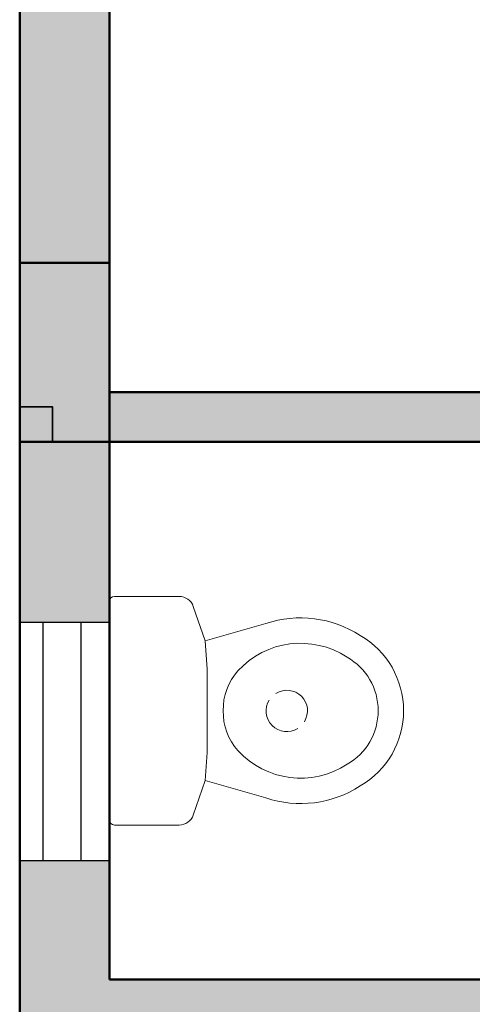
# Model space of a CAD drawing. Units: inches. Extents: x -7 to 1228, y -146 to 1091.
# Tile 7 of 88: x 60 to 105, y 276 to 375. Entities that reach past the tile are written whole.
import ezdxf

# ---------------------------------------------------------------- set-up
doc = ezdxf.new("R2010")
doc.units = ezdxf.units.IN
for name, color, linetype, lineweight in [('A-COLS', 6, 'Continuous', 35), ('A-FLOR-FIXT', 8, 'Continuous', 18), ('A-GLAZ', 175, 'Continuous', 25), ('A-WALL', 7, 'Continuous', 50), ('A-WALL-PATT', 251, 'Continuous', 13)]:
    doc.layers.add(name, color=color, linetype=linetype, lineweight=lineweight)

# ---------------------------------------------------------------- blocks, each defined once
blk = doc.blocks.new('A$C7B5C7CD4')
at = {"ltscale": 20}
for p, q in [((0, 0.614), (0, 0.4765)), ((0.243, 0.625), (0.011, 0.625)), ((0.243, 0.625), (0.475, 0.625)), ((0.486, 0.614), (0.486, 0.4765)), ((0.0212, 0.4467), (0.0946, 0.4214)), ((0.4648, 0.4467), (0.3914, 0.4214)), ((0.0946, 0.4214), (0.0576, 0.293)), ((0.0946, 0.4214), (0.1544, 0.4173)), ((0.3914, 0.4214), (0.3316, 0.4173)), ((0.3914, 0.4214), (0.4284, 0.293)), ((0.3316, 0.4173), (0.1544, 0.4173))]:
    blk.add_line(p, q, dxfattribs=at)
for centre, radius, start, end in [((0.011, 0.614), 0.011, 90, 180), ((0.475, 0.614), 0.011, 0, 90), ((0.0315, 0.4765), 0.0315, 180, 251), ((0.4545, 0.4765), 0.0315, 289, 0), ((0.24, 0.2602), 0.123, 88.6158, 131.7414), ((0.246, 0.2602), 0.123, 48.2586, 91.3842), ((0.2796, 0.219), 0.18, 132.4207, 213.289), ((0.2064, 0.219), 0.18, 326.711, 47.5793), ((0.2796, 0.219), 0.234, 161.5846, 212.8753), ((0.2064, 0.219), 0.234, 327.1247, 18.4154), ((0.243, 0.185), 0.131, 209.6292, 270), ((0.243, 0.185), 0.131, 270, 330.3708), ((0.243, 0.185), 0.185, 210.1745, 270), ((0.243, 0.185), 0.185, 270, 329.8255)]:
    blk.add_arc(centre, radius, start, end, dxfattribs=at)
for start, end in [(58.1785, 211.8215), (238.1785, 31.8215)]:
    blk.add_arc((0.2426, 0.2481), 0.0439, start, end)
blk = doc.blocks.new('WIN-24')
for p, q in [((0, 0), (0, 24)), ((0, 24), (9, 24)), ((2.343, 0), (2.343, 24)), ((2.343, 24), (6.137, 24)), ((6.137, 24), (6.137, 0)), ((9, 24), (9, 0)), ((9, 0), (0, 0))]:
    blk.add_line(p, q)

msp = doc.modelspace()

# ---------------------------------------------------------------- hatches: boundary and pattern name
at = {"layer": 'A-COLS'}
h = msp.add_hatch(color=256, dxfattribs=at)
h.dxf.hatch_style = 1
h.paths.add_polyline_path([(60, 336.546), (63.289, 336.546), (63.289, 333), (69, 333), (69, 351), (60, 351)])
h = msp.add_hatch(color=256, dxfattribs=at)
h.dxf.hatch_style = 1
h.paths.add_polyline_path([(60, 336.546), (60, 333), (63.289, 333), (63.289, 336.546)])
at = {"layer": 'A-WALL-PATT'}
h = msp.add_hatch(color=256, dxfattribs=at)
h.dxf.hatch_style = 1
h.paths.add_polyline_path([(69, 568), (60, 568), (60, 493), (63.289, 493), (69, 493)])
h.paths.add_polyline_path([(69, 662.405), (60, 662.405), (60, 586), (69, 586)], flags=17)
h.paths.add_polyline_path([(69, 723), (184, 723), (184, 734), (179, 734), (179, 728), (69, 728), (69, 741.623), (60, 741.623), (60, 698.405), (69, 698.405)], flags=17)
h.paths.add_polyline_path([(69, 782), (231, 782), (231, 728), (231, 723), (231, 586), (236, 586), (236, 787), (69, 787), (69, 800.126), (60, 800.126), (60, 765.623), (69, 765.623)])
h.paths.add_polyline_path([(184, 842), (189, 842), (189, 848), (173, 848), (173, 842), (179, 842), (179, 787), (184, 787)])
h.paths.add_polyline_path([(118.22, 69), (69, 69), (69, 60), (118.22, 60)])
h.paths.add_polyline_path([(227, 69), (154.22, 69), (154.22, 60), (227, 60)])
h.paths.add_polyline_path([(236, 60), (232.711, 60), (227, 60), (227, 36), (236, 36)])
h.paths.add_polyline_path([(389, 60), (380, 60), (380, 36), (389, 36)])
h.paths.add_polyline_path([(384, 181), (380, 181), (380, 115), (380, 78), (384, 78)])
h.paths.add_polyline_path([(380, 115), (334.547, 115), (334.547, 109), (380, 109)])
h.paths.add_polyline_path([(274.547, 115), (236, 115), (236, 201), (232.711, 201), (231, 201), (231, 78), (236, 78), (236, 109), (274.547, 109)])
h.paths.add_polyline_path([(69, 123), (60, 123), (60, 78), (69, 78)])
h.paths.add_polyline_path([(69, 201), (60, 201), (60, 159), (69, 159)])
h.paths.add_polyline_path([(143, 219), (69, 219), (69, 213), (143, 213)], flags=17)
h.paths.add_polyline_path([(189, 219), (184, 219), (184, 274), (231, 274), (231, 219), (236, 219), (236, 279), (184, 279), (184, 297), (179, 297), (179, 279), (69, 279), (69, 290.912), (60, 290.912), (60, 262.179), (69, 262.179), (69, 274), (179, 274), (179, 219), (173, 219), (173, 213), (189, 213)])
h.paths.add_polyline_path([(69, 238.179), (60, 238.179), (60, 219), (69, 219)], flags=17)
h.paths.add_polyline_path([(69, 333), (60, 333), (60, 314.912), (69, 314.912), (69, 316.965)])
h.paths.add_polyline_path([(190, 338), (184, 338), (69, 338), (69, 333), (179, 333), (179, 327), (184, 327), (184, 333.021), (190, 333.046)])
h.paths.add_polyline_path([(69, 386.806), (60, 386.806), (60, 351), (69, 351)])
h.paths.add_polyline_path([(69, 475), (60, 475), (60, 422.806), (69, 422.806)])
h.paths.add_polyline_path([(236, 475), (231, 475), (231, 351.238), (236, 351.238)])
h.paths.add_polyline_path([(384, 475), (380, 475), (380, 362), (384, 362)])
h.paths.add_polyline_path([(547, 307), (439, 307), (439, 356), (445, 356), (445, 362), (433, 362), (433, 307), (380, 307), (380, 244), (380, 241), (384, 241), (384, 301), (433, 301), (433, 277), (439, 277), (439, 301), (547, 301)])
h.paths.add_polyline_path([(547, 241), (439, 241), (439, 247), (433, 247), (433, 235), (547, 235)])
h.paths.add_polyline_path([(450, 69), (440.286, 69), (424.889, 69), (389, 69), (389, 60), (450, 60)])
h.paths.add_polyline_path([(547, 69), (486, 69), (486, 60), (547, 60)])
h.paths.add_polyline_path([(556, 148.268), (547, 148.268), (547, 78), (556, 78)])
h.paths.add_polyline_path([(556, 223), (547, 223), (547, 195), (547, 184.268), (556, 184.268)])
h.paths.add_polyline_path([(556, 311.192), (547, 311.192), (547, 273.075), (556, 273.075)])
h.paths.add_polyline_path([(556, 344), (552.711, 344), (547, 344), (547, 335.192), (556, 335.192)])
h.paths.add_polyline_path([(556, 249.075), (547, 249.075), (547, 241), (556, 241)])
h.paths.add_polyline_path([(547, 362), (475, 362), (475, 356), (547, 356)], flags=0)
h.paths.add_polyline_path([(556, 399.621), (547, 399.621), (547, 362), (556, 362)])
h.paths.add_polyline_path([(556, 475), (547, 475), (547, 435.621), (556, 435.621)])
h.paths.add_polyline_path([(547, 493), (389, 493), (389, 487), (547, 487)])
h.paths.add_polyline_path([(380, 493), (278, 493), (278, 487), (380, 487)])
h.paths.add_polyline_path([(227, 493), (69, 493), (69, 487), (227, 487)])
h.paths.add_polyline_path([(643, 122.445), (634, 122.445), (634, 78), (643, 78)])
h.paths.add_polyline_path([(702.5, 69), (692.786, 69), (677.389, 69), (643, 69), (643, 60), (702.5, 60)])
h.paths.add_polyline_path([(798, 69), (738.5, 69), (738.5, 60), (798, 60)])
h.paths.add_polyline_path([(807, 60), (803.711, 60), (798, 60), (798, 36), (807, 36)])
h.paths.add_polyline_path([(807, 109), (846.751, 109), (846.751, 115), (807, 115), (807, 159), (802, 159), (802, 78), (807, 78)])
h.paths.add_polyline_path([(807, 201), (802, 201), (802, 195), (807, 195)])
h.paths.add_polyline_path([(643, 201), (634, 201), (634, 158.445), (643, 158.445)])
h.paths.add_polyline_path([(756, 225), (751, 225), (751, 219), (643, 219), (643, 213), (756, 213)])
h.paths.add_polyline_path([(643, 240.848), (634, 240.848), (634, 219), (643, 219)])
h.paths.add_polyline_path([(643, 274), (643, 288.629), (634, 288.629), (634, 264.848), (643, 264.848)])
h.paths.add_polyline_path([(802, 279), (756, 279), (756, 297), (751, 297), (751, 279), (643, 279), (643, 274), (751, 274), (751, 255), (756, 255), (756, 274), (802, 274)])
h.paths.add_polyline_path([(807, 333), (803.711, 333), (802, 333), (802, 279), (802, 274), (802, 219), (807, 219)])
h.paths.add_polyline_path([(956, 182), (951, 182), (951, 115), (906.751, 115), (906.751, 109), (951, 109), (951, 78), (956, 78)])
h.paths.add_polyline_path([(960, 60), (951, 60), (951, 36), (960, 36)])
h.paths.add_polyline_path([(1021, 69), (1005.781, 69), (960, 69), (960, 60), (1021, 60)])
h.paths.add_polyline_path([(956, 224), (951, 224), (951, 218), (956, 218)])
h.paths.add_polyline_path([(956, 302), (1004, 302), (1004, 278), (1010, 278), (1010, 302), (1118, 302), (1118, 290.809), (1127, 290.809), (1127, 326.968), (1118, 326.968), (1118, 320.966), (1118, 307), (1010, 307), (1010, 356), (1016, 356), (1016, 362), (1004, 362), (1004, 307), (951, 307), (951, 244), (951, 242), (954.289, 242), (956, 242)])
h.paths.add_polyline_path([(643, 333), (634, 333), (634, 312.629), (643, 312.629), (643, 316.965)])
h.paths.add_polyline_path([(756, 338), (643, 338), (643, 333), (751, 333), (751, 327), (756, 327)])
h.paths.add_polyline_path([(643, 388), (634, 388), (634, 351), (643, 351)])
h.paths.add_polyline_path([(807, 357), (802, 357), (802, 351), (807, 351)])
h.paths.add_polyline_path([(807, 475), (802, 475), (802, 393), (807, 393)])
h.paths.add_polyline_path([(643, 475), (634, 475), (634, 424), (643, 424)])
h.paths.add_polyline_path([(798, 493), (643, 493), (643, 487), (798, 487)])
h.paths.add_polyline_path([(634, 493), (556, 493), (556, 487), (634, 487)])
h.paths.add_polyline_path([(813, 493), (807, 493), (807, 487), (813, 487)])
h.paths.add_polyline_path([(951, 493), (849, 493), (849, 487), (951, 487)])
h.paths.add_polyline_path([(956, 484), (951, 484), (951, 374), (956, 374)])
h.paths.add_polyline_path([(1109, 493), (969, 493), (969, 487), (1109, 487)])
h.paths.add_polyline_path([(1127, 484), (1118, 484), (1118, 450.641), (1127, 450.641)])
h.paths.add_polyline_path([(1127, 414.641), (1118, 414.641), (1118, 365), (1127, 365)])
h.paths.add_polyline_path([(1109, 362), (1046, 362), (1046, 356), (1109, 356)], flags=17)
h.paths.add_polyline_path([(1127, 356), (1123.454, 356), (1118, 356), (1118, 350.968), (1127, 350.968)], flags=0)
h.paths.add_polyline_path([(1127, 266.809), (1118, 266.809), (1118, 262.361), (1118, 242), (1127, 242)], flags=17)
h.paths.add_polyline_path([(1118, 242), (1010, 242), (1010, 248), (1004, 248), (1004, 237), (1118, 237)])
h.paths.add_polyline_path([(1127, 224), (1118, 224), (1118, 170), (1127, 170)])
h.paths.add_polyline_path([(1127, 134), (1118, 134), (1118, 78), (1127, 78)])
h.paths.add_polyline_path([(1118, 69), (1057, 69), (1057, 60), (1118, 60)])
h.paths.add_polyline_path([(227, 571.546), (227, 574), (69, 574), (69, 568), (227, 568)])
h.paths.add_polyline_path([(380, 571.546), (380, 574), (278, 574), (278, 568), (380, 568)])
h.paths.add_polyline_path([(242, 574), (236, 574), (236, 568), (242, 568)])
h.paths.add_polyline_path([(547, 571.546), (547, 574), (389, 574), (389, 568), (547, 568)])
h.paths.add_polyline_path([(384, 733), (380, 733), (380, 586), (384, 586)])
h.paths.add_polyline_path([(556, 646), (634, 646), (634, 655), (547, 655), (547, 586), (556, 586)])
h.paths.add_polyline_path([(634, 574), (556, 574), (556, 568), (634, 568)])
h.paths.add_polyline_path([(643, 655), (634, 655), (634, 586), (643, 586)])
h.paths.add_polyline_path([(798, 574), (643, 574), (643, 568), (798, 568)])
h.paths.add_polyline_path([(643, 663.854), (634, 663.854), (634, 655), (643, 655)])
h.paths.add_polyline_path([(556, 676.967), (547, 676.967), (547, 655), (556, 655)])
h.paths.add_polyline_path([(556, 733), (547, 733), (547, 712.967), (556, 712.967)])
h.paths.add_polyline_path([(643, 710), (634, 710), (634, 699.854), (643, 699.854)])
h.paths.add_polyline_path([(807, 668), (802, 668), (802, 586), (807, 586)])
h.paths.add_polyline_path([(951, 574), (849, 574), (849, 568), (951, 568)])
h.paths.add_polyline_path([(956, 691), (951, 691), (951, 577), (956, 577)])
h.paths.add_polyline_path([(1109, 574), (969, 574), (969, 568), (1109, 568)])
h.paths.add_polyline_path([(1127, 643.403), (1118, 643.403), (1118, 577), (1127, 577)])
h.paths.add_polyline_path([(1127, 568), (1123.454, 568), (1118, 568), (1118, 493), (1127, 493)])
h.paths.add_polyline_path([(1127, 733), (1118, 733), (1118, 679.403), (1127, 679.403)])
h.paths.add_polyline_path([(1127, 777.348), (1118, 777.348), (1118, 770.035), (1118, 751), (1127, 751)], flags=17)
h.paths.add_polyline_path([(1118, 751), (1010, 751), (1010, 757), (1004, 757), (1004, 745), (1118, 745)])
h.paths.add_polyline_path([(956, 811), (1004, 811), (1004, 787), (1010, 787), (1010, 811), (1017.874, 811), (1017.874, 811.627, -0.414214), (1018.247, 812), (1031.978, 812, -0.414214), (1032.351, 811.627), (1032.351, 811), (1118, 811), (1118, 801.348), (1127, 801.348), (1127, 834.685), (1118, 834.685), (1118, 830.238), (1118, 817), (1010, 817), (1010, 866), (1016, 866), (1016, 872), (1004, 872), (1004, 817), (956, 817), (956, 866), (951, 866), (951, 751), (954.289, 751), (956, 751)])
h.paths.add_polyline_path([(1118, 872), (1046, 872), (1046, 866), (1118, 866)], flags=17)
h.paths.add_polyline_path([(1127, 924.711), (1118, 924.711), (1118, 884), (1127, 884)])
h.paths.add_polyline_path([(1127, 866), (1123.711, 866), (1118, 866), (1118, 858.685), (1127, 858.685)], flags=17)
h.paths.add_polyline_path([(956, 983), (951, 983), (951, 952), (807, 952), (807, 983), (802, 983), (802, 902), (807, 902), (807, 946), (951, 946), (951, 884), (956, 884)])
h.paths.add_polyline_path([(807, 842), (802, 842), (802, 787), (756, 787), (756, 806), (751, 806), (751, 787), (643, 787), (643, 782), (751, 782), (751, 764), (756, 764), (756, 782), (802, 782), (802, 728), (807, 728)])
h.paths.add_polyline_path([(756, 848), (643, 848), (643, 842), (751, 842), (751, 836), (756, 836)])
h.paths.add_polyline_path([(756, 734), (751, 734), (751, 728), (643, 728), (643, 723), (756, 723)])
h.paths.add_polyline_path([(643, 749.791), (634, 749.791), (634, 728), (637.289, 728), (643, 728)])
h.paths.add_polyline_path([(643, 805.405), (634, 805.405), (634, 773.791), (643, 773.791)])
h.paths.add_polyline_path([(643, 896.663), (634, 896.663), (634, 860), (637.289, 860), (643, 860)])
h.paths.add_polyline_path([(643, 842), (634, 842), (634, 829.405), (643, 829.405)])
h.paths.add_polyline_path([(643, 983), (634, 983), (634, 932.663), (643, 932.663)])
h.paths.add_polyline_path([(1127, 983), (1118, 983), (1118, 960.711), (1127, 960.711)])
h.paths.add_polyline_path([(1118, 1001), (1077.525, 1001), (1077.525, 992), (1118, 992)])
h.paths.add_polyline_path([(1041.525, 1001), (960, 1001), (960, 992), (1041.525, 992)])
h.paths.add_polyline_path([(960, 1025), (951, 1025), (951, 1001), (954.289, 1001), (960, 1001)])
h.paths.add_polyline_path([(807, 1025), (798, 1025), (798, 1001), (807, 1001)])
h.paths.add_polyline_path([(798, 1001), (738.5, 1001), (738.5, 992), (798, 992)])
h.paths.add_polyline_path([(702.5, 1001), (643, 1001), (643, 992), (702.5, 992)])
h.paths.add_polyline_path([(547, 1001), (499.113, 1001), (499.113, 992), (547, 992)])
h.paths.add_polyline_path([(463.113, 1001), (389, 1001), (389, 992), (463.113, 992)])
h.paths.add_polyline_path([(389, 1025), (380, 1025), (380, 1022), (380, 1001), (383.289, 1001), (389, 1001)])
h.paths.add_polyline_path([(236, 1025), (227, 1025), (227, 1001), (236, 1001)])
h.paths.add_polyline_path([(236, 983), (231, 983), (231, 860), (236, 860)])
h.paths.add_polyline_path([(274.547, 952), (236, 952), (236, 946), (274.547, 946)])
h.paths.add_polyline_path([(380, 952), (334.547, 952), (334.547, 946), (380, 946)])
h.paths.add_polyline_path([(384, 983), (380, 983), (380, 884), (383.289, 884), (384, 884)])
h.paths.add_polyline_path([(227, 1001), (155.012, 1001), (155.012, 992), (162.875, 992), (227, 992)])
h.paths.add_polyline_path([(119.012, 1001), (69, 1001), (69, 992), (119.012, 992)])
h.paths.add_polyline_path([(69, 983), (60, 983), (60, 922.987), (69, 922.987)])
h.paths.add_polyline_path([(69, 886.987), (60, 886.987), (60, 860), (63.289, 860), (69, 860)])
h.paths.add_polyline_path([(143, 848), (69, 848), (69, 842), (143, 842)])

# ---------------------------------------------------------------- linework, layer by layer
at = {"layer": 'A-COLS'}
msp.add_lwpolyline([(60, 333), (63.289, 333), (63.289, 336.546), (60, 336.546)], close=True, dxfattribs=at)
at = {"layer": 'A-WALL'}
for p, q in [((60, 1001), (60, 60)), ((69, 568), (69, 279)), ((69, 338), (69, 487)), ((69, 351), (60, 351)), ((60, 351), (60, 333)), ((69, 333), (69, 351)), ((184, 338), (69, 338)), ((60, 333), (69, 333)), ((179, 333), (69, 333)), ((69, 279), (69, 333)), ((179, 279), (69, 279))]:
    msp.add_line(p, q, dxfattribs=at)

# ---------------------------------------------------------------- block references
at = {"layer": 'A-FLOR-FIXT', "xscale": 47.26153857112405, "yscale": 47.26153857112405, "zscale": 47.26153857112405, "rotation": 90}
msp.add_blockref('A$C7B5C7CD4', (98.538, 294.515), dxfattribs=at)
at = {"layer": 'A-GLAZ'}
msp.add_blockref('WIN-24', (60, 290.911), dxfattribs=at)

doc.saveas('drawing.dxf')
